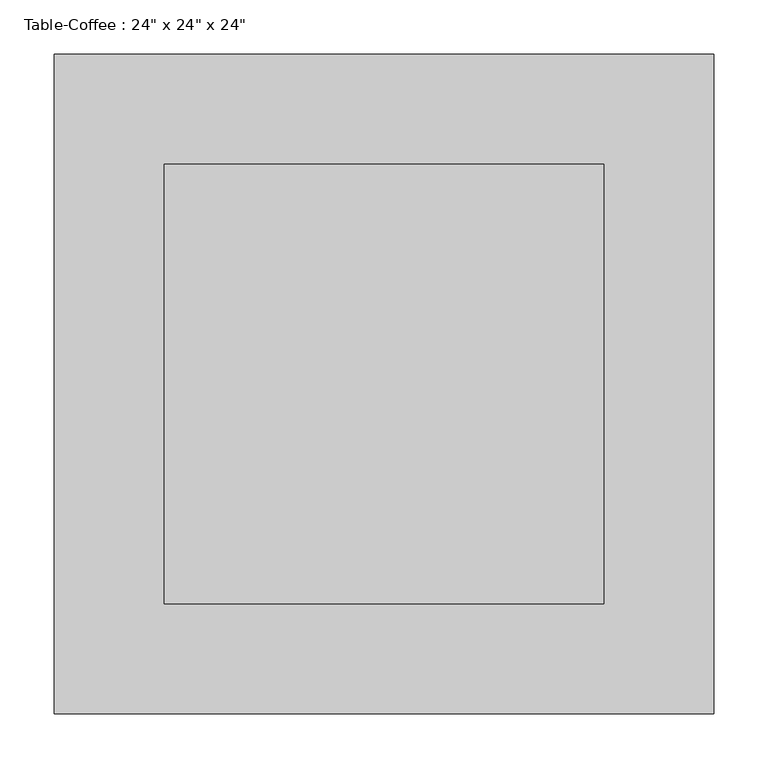
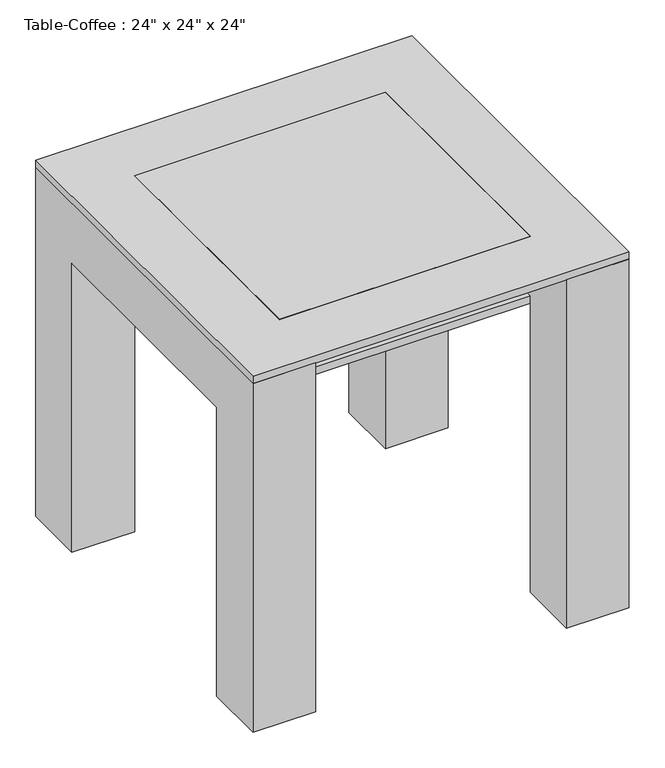
"""IFC4 building model written with IfcOpenShell, lengths in millimetres: furniture geometry."""

from ifc_helpers import new_model, si_unit, frame, origin, place, context, project, spatial, polyline, outline, extrude, source, transform, mapped, element, save


def furniture_b5c51a22(model_context):
    return source(origin(), model_context, "Body", "SweptSolid", [
        extrude(outline(polyline([(221.4657667, 298.4110778), (221.4657667, -107.9889222), (-184.9342333, -107.9889222), (-184.9342333, 298.4110778), (221.4657667, 298.4110778)])), frame((0.0, 0.0, 495.3), z_axis=(0.0, 0.0, 1.0), x_axis=(1.0, 0.0, 0.0)), (0.0, 0.0, 1.0), 12.7),
        extrude(outline(polyline([(400.0110778, 0.0), (298.4110778, 0.0), (298.4110778, 495.3), (-107.9889222, 495.3), (-107.9889222, 0.0), (-209.5889222, 0.0), (-209.5889222, 596.9), (400.0110778, 596.9), (400.0110778, 0.0)])), frame((221.4657667, 0.0, 0.0), z_axis=(1.0, 0.0, 0.0), x_axis=(0.0, 1.0, 0.0)), (0.0, 0.0, 1.0), 101.6),
        extrude(outline(polyline([(400.0110778, 596.9), (400.0110778, 0.0), (298.4110778, 0.0), (298.4110778, 495.3), (-107.9889222, 495.3), (-107.9889222, 0.0), (-209.5889222, 0.0), (-209.5889222, 596.9), (400.0110778, 596.9)])), frame((-286.5342333, 0.0, 0.0), z_axis=(1.0, 0.0, 0.0), x_axis=(0.0, 1.0, 0.0)), (0.0, 0.0, 1.0), 101.6),
        extrude(outline(polyline([(221.4657667, 298.4110778), (221.4657667, -107.9889222), (-184.9342333, -107.9889222), (-184.9342333, 298.4110778), (221.4657667, 298.4110778)])), frame((0.0, 0.0, 596.9), z_axis=(0.0, 0.0, 1.0), x_axis=(1.0, 0.0, 0.0)), (0.0, 0.0, 1.0), 12.7),
        extrude(outline(polyline([(323.0657667, 400.0110778), (323.0657667, -209.5889222), (-286.5342333, -209.5889222), (-286.5342333, 400.0110778), (323.0657667, 400.0110778)]), holes=[polyline([(221.4657667, 298.4110778), (-184.9342333, 298.4110778), (-184.9342333, -107.9889222), (221.4657667, -107.9889222), (221.4657667, 298.4110778)])]), frame((0.0, 0.0, 596.9), z_axis=(0.0, 0.0, 1.0), x_axis=(1.0, 0.0, 0.0)), (0.0, 0.0, 1.0), 12.7),
    ])


if __name__ == "__main__":
    model = new_model("IFC4")
    model_context = context("Model", 3, world=origin())
    ifc_project = project(units=[si_unit("LENGTHUNIT", "METRE", prefix="MILLI")], contexts=[model_context])
    site = spatial("IfcSite", under=ifc_project)
    building = spatial("IfcBuilding", under=site)
    placement = place(None, origin())
    furniture_shape = furniture_b5c51a22(model_context)
    element("IfcFurniture", 1, ObjectType="Table-Coffee : 24\" x 24\" x 24\"", at=placement, inside=building, context=model_context, shape_type="MappedRepresentation", body=[
        mapped(furniture_shape, transform((0.0, 0.0, 0.0), x_axis=(1.0, 0.0, 0.0), y_axis=(0.0, 1.0, 0.0), z_axis=(0.0, 0.0, 1.0))),
    ])
    save(model, "model.ifc")

# Revit data of these elements
# Type "Table-Coffee : 24\" x 24\" x 24\""
#   Assembly Code = "E2020200"
#   Height = 2' - 0"
#   Length = 2' - 0"
#   Width = 2' - 0"
#   Top Material = Paper
#   Frame Material = none
#   Default Elevation = 0
# Element 1 (IfcFurniture, "Table-Coffee : 24\" x 24\" x 24\"")
#   Materials on its faces: "Paper", "Glass - Clear, Grey"
# Materials
#   "Paper": class "Generic", colour RGB 0 0 0, transparency 0, Description = "Paper", Cost = 0
#   "Glass - Clear, Grey": class "Glass", colour RGB 252 255 255, transparency 0.64
